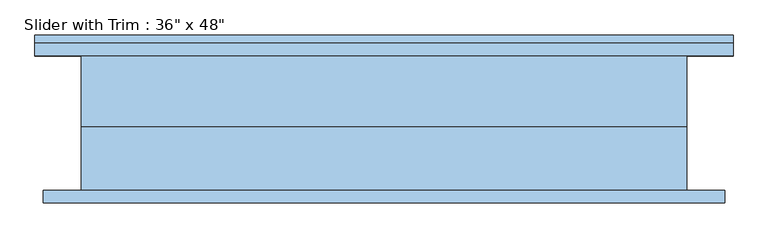
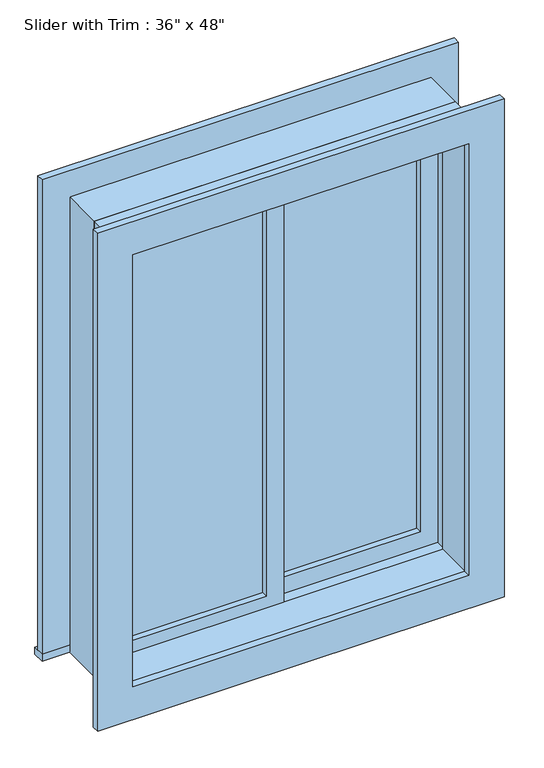
"""IFC4 building model written with IfcOpenShell, lengths in millimetres: window geometry."""

from ifc_helpers import new_model, si_unit, frame, origin, place, context, project, spatial, polyline, outline, extrude, source, transform, mapped, element, save


def window_54100e87(model_context):
    return source(origin(), model_context, "Body", "SweptSolid", [
        extrude(outline(polyline([(-393.7, 22.225), (-22.225, 22.225), (-22.225, 9.525), (-393.7, 9.525), (-393.7, 22.225)])), frame((0.0, 0.0, 977.9), z_axis=(0.0, 0.0, 1.0), x_axis=(1.0, 0.0, 0.0)), (0.0, 0.0, 1.0), 1092.2),
        extrude(outline(polyline([(2114.55, -438.15), (933.45, -438.15), (933.45, 22.225), (2114.55, 22.225), (2114.55, -438.15)]), holes=[polyline([(2070.1, -393.7), (2070.1, -22.225), (977.9, -22.225), (977.9, -393.7), (2070.1, -393.7)])]), frame((0.0, -6.35, 0.0), z_axis=(0.0, 1.0, 0.0), x_axis=(0.0, 0.0, 1.0)), (0.0, 0.0, 1.0), 44.45),
        extrude(outline(polyline([(-527.05, 133.35), (527.05, 133.35), (527.05, 101.6), (-527.05, 101.6), (-527.05, 133.35)])), frame((0.0, 0.0, 914.4), z_axis=(0.0, 0.0, 1.0), x_axis=(1.0, 0.0, 0.0)), (0.0, 0.0, 1.0), 19.05),
        extrude(outline(polyline([(2114.55, -438.15), (2114.55, 438.15), (933.45, 438.15), (933.45, 527.05), (2203.45, 527.05), (2203.45, -527.05), (933.45, -527.05), (933.45, -438.15), (2114.55, -438.15)])), frame((0.0, 101.6, 0.0), z_axis=(0.0, 1.0, 0.0), x_axis=(0.0, 0.0, 1.0)), (0.0, 0.0, 1.0), 19.05),
        extrude(outline(polyline([(2190.75, 514.35), (2190.75, -514.35), (857.25, -514.35), (857.25, 514.35), (2190.75, 514.35)]), holes=[polyline([(2101.85, 425.45), (946.15, 425.45), (946.15, -425.45), (2101.85, -425.45), (2101.85, 425.45)])]), frame((0.0, -120.65, 0.0), z_axis=(0.0, 1.0, 0.0), x_axis=(0.0, 0.0, 1.0)), (0.0, 0.0, 1.0), 19.05),
        extrude(outline(polyline([(393.7, 53.975), (22.225, 53.975), (22.225, 66.675), (393.7, 66.675), (393.7, 53.975)])), frame((0.0, 0.0, 977.9), z_axis=(0.0, 0.0, 1.0), x_axis=(1.0, 0.0, 0.0)), (0.0, 0.0, 1.0), 1092.2),
        extrude(outline(polyline([(2114.55, -22.225), (933.45, -22.225), (933.45, 438.15), (2114.55, 438.15), (2114.55, -22.225)]), holes=[polyline([(2070.1, 22.225), (2070.1, 393.7), (977.9, 393.7), (977.9, 22.225), (2070.1, 22.225)])]), frame((0.0, 38.1, 0.0), z_axis=(0.0, 1.0, 0.0), x_axis=(0.0, 0.0, 1.0)), (0.0, 0.0, 1.0), 44.45),
        extrude(outline(polyline([(2133.6, -457.2), (914.4, -457.2), (914.4, 457.2), (2133.6, 457.2), (2133.6, -457.2)]), holes=[polyline([(2101.85, -425.45), (2101.85, 425.45), (946.15, 425.45), (946.15, -425.45), (2101.85, -425.45)])]), frame((0.0, -101.6, 0.0), z_axis=(0.0, 1.0, 0.0), x_axis=(0.0, 0.0, 1.0)), (0.0, 0.0, 1.0), 95.25),
        extrude(outline(polyline([(2133.6, 457.2), (2133.6, -457.2), (914.4, -457.2), (914.4, 457.2), (2133.6, 457.2)]), holes=[polyline([(2114.55, 438.15), (933.45, 438.15), (933.45, -438.15), (2114.55, -438.15), (2114.55, 438.15)])]), frame((0.0, -6.35, 0.0), z_axis=(0.0, 1.0, 0.0), x_axis=(0.0, 0.0, 1.0)), (0.0, 0.0, 1.0), 107.95),
    ])


if __name__ == "__main__":
    model = new_model("IFC4")
    model_context = context("Model", 3, world=origin())
    ifc_project = project(units=[si_unit("LENGTHUNIT", "METRE", prefix="MILLI")], contexts=[model_context])
    site = spatial("IfcSite", under=ifc_project)
    building = spatial("IfcBuilding", under=site)
    placement = place(None, origin())
    window_shape = window_54100e87(model_context)
    element("IfcWindow", 1, ObjectType="Slider with Trim : 36\" x 48\"", at=placement, inside=building, context=model_context, shape_type="MappedRepresentation", body=[
        mapped(window_shape, transform((0.0, 0.0, 0.0), x_axis=(1.0, 0.0, 0.0), y_axis=(0.0, 1.0, 0.0), z_axis=(0.0, 0.0, 1.0))),
    ])
    save(model, "model.ifc")

# Revit data of these elements
# Type "Slider with Trim : 36\" x 48\""
#   Type Mark = "11"
#   Construction Type Id = "GSP4R"
#   Assembly Code = "B2020100"
#   Analytic Construction = "1/8 in Pilkington single glazing"
#   Visual Light Transmittance = 0.9
#   Solar Heat Gain Coefficient = 0.78
#   Heat Transfer Coefficient (U) = 3.6886 W/(m²·K)
#   Height = 4' - 0"
#   Default Sill Height = 3' - 0"
#   Trim Projection - Ext. = 0' - 0 3/4"
#   Trim Projection - Int. = 0' - 0 3/4"
#   Trim Width - Exterior = 0' - 3 1/2"
#   Trim Width - Interior = 0' - 3 1/2"
#   Width = 3' - 0"
#   Window Inset = 0' - 0 3/4"
#   Glass Pane Material = Glass
#   Sash Material = Iron, Ductile
#   Trim Exterior Material = Iron, Ductile
#   Trim Interior Material = Iron, Ductile
#   Wall Closure = (empty or 0)
# Element 1 (IfcWindow, "Slider with Trim : 36\" x 48\"")
#   Materials on its faces: "Iron, Ductile", "Glass"
# Materials
#   "Glass": class "Glass", colour RGB 0 128 192, transparency 0.75, Description = "Soda Lime Glass", Cost = 0
#   "Iron, Ductile": class "Metal", colour RGB 0 0 0, transparency 0, Description = "Ductile cast iron", Cost = 0
